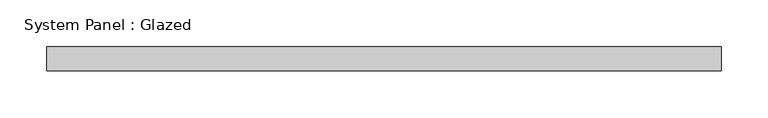
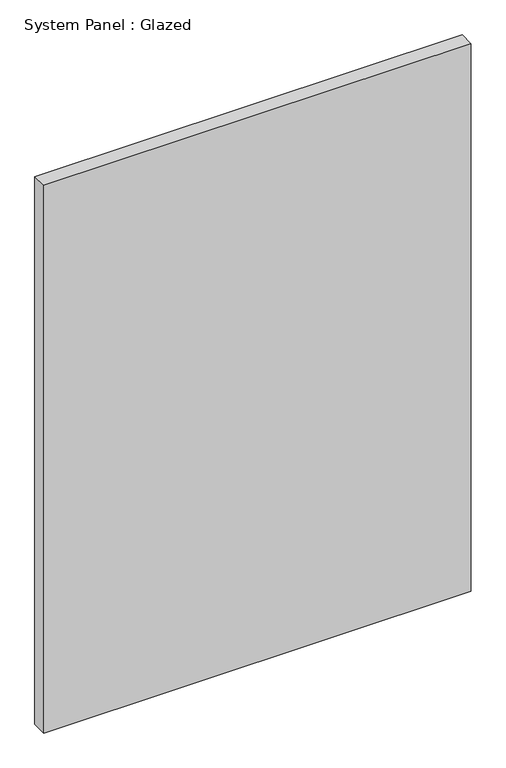
"""IFC4 building model written with IfcOpenShell, lengths in millimetres: plate geometry, System Panel : Glazed."""

from ifc_helpers import new_model, si_unit, origin, origin_with_axes, place, context, project, spatial, polyline, outline, extrude, source, transform, mapped, element, save


def system_panel_glazed_a527b3ca(model_context):
    return source(origin(), model_context, "Body", "SweptSolid", [
        extrude(outline(polyline([(358.775, 19.05), (-358.775, 19.05), (-358.775, 44.45), (358.775, 44.45), (358.775, 19.05)])), origin_with_axes(), (0.0, 0.0, 1.0), 971.55),
    ])


if __name__ == "__main__":
    model = new_model("IFC4")
    model_context = context("Model", 3, world=origin())
    ifc_project = project(units=[si_unit("LENGTHUNIT", "METRE", prefix="MILLI")], contexts=[model_context])
    site = spatial("IfcSite", under=ifc_project)
    building = spatial("IfcBuilding", under=site)
    placement = place(None, origin())
    system_panel_glazed_shape = system_panel_glazed_a527b3ca(model_context)
    element("IfcPlate", 1, ObjectType="System Panel : Glazed", at=placement, inside=building, context=model_context, shape_type="MappedRepresentation", body=[
        mapped(system_panel_glazed_shape, transform((0.0, 0.0, 0.0), x_axis=(1.0, 0.0, 0.0), y_axis=(0.0, 1.0, 0.0), z_axis=(0.0, 0.0, 1.0))),
    ])
    save(model, "model.ifc")

# Revit data of these elements
# Type "System Panel : Glazed"
#   Construction Type Id = "GSP4R"
#   Analytic Construction = "1/8 in Pilkington single glazing"
#   Visual Light Transmittance = 0.9
#   Solar Heat Gain Coefficient = 0.86
#   Heat Transfer Coefficient (U) = 1.18115 BTU/(h·ft²·°F)
#   Define Thermal Properties by = 1
# Element 1 (IfcPlate, "System Panel : Glazed")
#   Materials on its faces: "Glass"
# Materials
#   "Glass": class "Glass", colour RGB 0 128 192, transparency 0.75, Description = "Soda Lime Glass", Cost = 0
